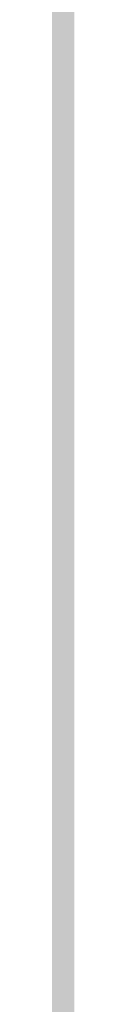
# Model space of a CAD drawing. Units: inches. Extents: x 2083 to 3317, y 1141 to 2115.
# Tile 191 of 256: x 3126.9559 to 3126.9582, y 1263.3548 to 1263.6134. Entities that reach past the tile are written whole.
import ezdxf

# ---------------------------------------------------------------- set-up
doc = ezdxf.new("R2010")
doc.units = ezdxf.units.IN
doc.layers.add('A-ANNO-DIMS', color=2, linetype='Continuous', lineweight=18)
doc.layers.add('A-WALL-PATT', color=251, linetype='Continuous', lineweight=13, true_color=0x636466)
doc.styles.get("Standard").update_dxf_attribs({"font": 'arial.ttf'})
doc.dimstyles.new('ISO-25', dxfattribs={"dimtxt": 12, "dimasz": 12, "dimexe": 1.25, "dimexo": 0.625, "dimtad": 1, "dimlunit": 3, "dimtxsty": 'Standard', "dimcen": 2.5, "dimadec": 0, "dimazin": 0, "dimtfac": 1, "dimtmove": 0, "dimatfit": 3, "dimfxl": 1, "dimarcsym": 0})

# ---------------------------------------------------------------- blocks, each defined once
blk = doc.blocks.new('*D26')
at = {"layer": 'A-ANNO-DIMS', "color": 0, "lineweight": -2, "transparency": 16777216}
for p, q in [((3088.98584, 1274.91509), (3088.98584, 1270.95196)), ((3111.24004, 1274.91509), (3111.24004, 1270.95196)), ((3076.98584, 1272.20196), (2840.26245, 1272.20196)), ((3111.24004, 1272.20196), (3088.98584, 1272.20196)), ((3123.24004, 1272.20196), (3135.24004, 1272.20196))]:
    blk.add_line(p, q, dxfattribs=at)
at = {"layer": 'A-ANNO-DIMS', "color": 0, "transparency": 16777216}
for points in [[(3076.98584, 1274.20196), (3076.98584, 1270.20196), (3088.98584, 1272.20196)], [(3123.24004, 1274.20196), (3123.24004, 1270.20196), (3111.24004, 1272.20196)]]:
    blk.add_solid(points, dxfattribs=at)
at = {"layer": 'Defpoints', "color": 0, "transparency": 16777216}
for p in [(3088.98584, 1275.54009), (3111.24004, 1275.54009), (3088.98584, 1272.20196)]:
    blk.add_point(p, dxfattribs=at)
at = {"layer": 'A-ANNO-DIMS', "color": 0, "transparency": 16777216, "insert": (2952.62415, 1279.0316), "char_height": 12, "attachment_point": 5}
blk.add_mtext('NIGHTSTAND 1\'-10 1/2" TYP.', dxfattribs=at)
blk = doc.blocks.new('*D27')
at = {"layer": 'A-ANNO-DIMS', "color": 0, "lineweight": -2, "transparency": 16777216}
for p, q in [((3114.57817, 1309.79428), (3114.57817, 1321.79428)), ((3111.86504, 1297.79428), (3115.82817, 1297.79428)), ((3114.57817, 1297.79428), (3114.57817, 1275.54009)), ((3111.86504, 1275.54009), (3115.82817, 1275.54009)), ((3114.57817, 1263.54009), (3114.57817, 1140.98859))]:
    blk.add_line(p, q, dxfattribs=at)
at = {"layer": 'A-ANNO-DIMS', "color": 0, "transparency": 16777216}
for points in [[(3112.57817, 1309.79428), (3116.57817, 1309.79428), (3114.57817, 1297.79428)], [(3112.57817, 1263.54009), (3116.57817, 1263.54009), (3114.57817, 1275.54009)]]:
    blk.add_solid(points, dxfattribs=at)
at = {"layer": 'Defpoints', "color": 0, "transparency": 16777216}
for p in [(3111.24004, 1297.79428), (3111.24004, 1275.54009), (3114.57817, 1275.54009)]:
    blk.add_point(p, dxfattribs=at)
at = {"layer": 'A-ANNO-DIMS', "color": 0, "transparency": 16777216, "insert": (3107.74853, 1196.26434), "char_height": 12, "attachment_point": 5, "rotation": 90}
blk.add_mtext('1\'-10 1/2" TYP.', dxfattribs=at)

msp = doc.modelspace()

# ---------------------------------------------------------------- hatches: boundary and pattern name
at = {"layer": 'A-WALL-PATT'}
h = msp.add_hatch(color=256, dxfattribs=at)
h.dxf.hatch_style = 1
h.paths.add_polyline_path([(3126.95978, 2020.76136), (2748.95978, 2020.76136), (2604.95978, 2020.76136), (2226.95978, 2020.76136), (2226.95978, 1702.76136), (2466.95978, 1702.76136), (2466.95978, 1582.76136), (2418.95978, 1582.76136), (2418.95978, 1477.76136), (2226.95978, 1477.76136), (2226.95978, 1263.26136), (2544.95978, 1263.26136), (2544.95978, 1411.76136), (2604.95978, 1411.76136), (2685.95978, 1411.76136), (2685.95978, 1420.76136), (2604.95978, 1420.76136), (2604.95978, 1573.76136), (2604.95978, 1702.76136), (2604.95978, 2011.76136), (2748.95978, 2011.76136), (2748.95978, 1702.76136), (2862.95978, 1702.76136), (2862.95978, 1621.76136), (2871.95978, 1621.76136), (2871.95978, 1702.76136), (2883.95978, 1702.76136), (2883.95978, 1706.93946, -0.026459), (2883.95978, 1711.76136), (2757.95978, 1711.76136), (2757.95978, 1807.76136), (2787.95978, 1807.76136), (2787.95978, 1812.26136), (2757.95978, 1812.26136), (2757.95978, 2011.76136), (2877.95978, 2011.76136), (2877.95978, 1812.26136), (2847.95978, 1812.26136), (2847.95978, 1807.76136), (2889.83574, 1807.76136), (2889.83574, 1812.26136), (2882.45978, 1812.26136), (2882.45978, 2011.76136), (3117.95978, 2011.76136), (3117.95978, 1812.26136), (2937.83574, 1812.26136), (2937.83574, 1807.76136), (2995.70978, 1807.76136), (2995.70978, 1796.11767), (3000.20978, 1796.11767), (3000.20978, 1807.76136), (3117.95978, 1807.76136), (3117.95978, 1711.76136), (3000.20978, 1711.76136), (3000.20978, 1760.11767), (2998.5727, 1760.11767, -0.020711), (2995.70978, 1760.11767), (2995.70978, 1711.76136), (2931.95978, 1711.76136), (2931.95978, 1702.76136), (3126.95978, 1702.76136)])
h.paths.add_polyline_path([(2471.45978, 2011.76136), (2471.45978, 1810.01136), (2462.71694, 1810.01136), (2462.71694, 1805.51136), (2505.95978, 1805.51136), (2505.95978, 1810.01136), (2475.95978, 1810.01136), (2475.95978, 2011.76136), (2595.95978, 2011.76136), (2595.95978, 1810.01136), (2565.95978, 1810.01136), (2565.95978, 1805.51136), (2595.95978, 1805.51136), (2595.95978, 1711.76136), (2235.95978, 1711.76136), (2235.95978, 1805.51136), (2353.70978, 1805.51136), (2353.70978, 1796.05416), (2358.20978, 1796.05416), (2358.20978, 1805.51136), (2414.71694, 1805.51136), (2414.71694, 1810.01136), (2235.95978, 1810.01136), (2235.95978, 2011.76136)], flags=16)
h.paths.add_polyline_path([(2270.20473, 1994.61001), (2270.20473, 1970.61001), (2246.20473, 1970.61001), (2246.20473, 1994.61001)], flags=0)
edge = h.paths.add_edge_path(flags=0)
edge.add_ellipse((2332.02739, 1899.79818), major_axis=(-3.04299, 3.04299), ratio=0.1682525, start_angle=-161.33217, end_angle=-156.30711, ccw=False)
edge.add_ellipse((2333.08204, 1898.74353), major_axis=(-1.05465, 1.05465), ratio=0.4535321, start_angle=-123.37102, end_angle=-94.15911)
edge = h.paths.add_edge_path(flags=0)
edge.add_ellipse((2332.02739, 1968.87629), major_axis=(3.04299, 3.04299), ratio=0.1682525, start_angle=18.66783, end_angle=23.69289)
edge.add_spline(control_points=[(2332.9256, 1970.6911), (2332.22677, 1970.3361), (2330.89371, 1969.65891), (2328.41308, 1970.93214), (2327.20393, 1967.74871), (2324.7096, 1969.95559), (2322.53282, 1967.01235), (2320.01285, 1971.29581), (2317.68031, 1968.15784), (2316.04053, 1967.10205), (2315.4269, 1966.8096)], knot_values=[0, 0, 0, 0, 2.267059, 4.324559, 6.685584, 8.878641, 11.121502, 14.300359, 17.755284, 19.732645, 19.732645, 19.732645, 19.732645], degree=3, periodic=0)
edge.add_ellipse((2332.02739, 1968.87629), major_axis=(3.04299, 3.04299), ratio=0.1682525, start_angle=18.66783, end_angle=23.69289, ccw=False)
edge.add_ellipse((2333.08204, 1969.93094), major_axis=(1.05465, 1.05465), ratio=0.4535321, start_angle=56.62898, end_angle=85.84089, ccw=False)
edge = h.paths.add_edge_path(flags=0)
edge.add_spline(control_points=[(2296.42829, 1967.98791), (2293.6278, 1965.33631), (2287.70362, 1959.72709), (2299.74386, 1949.9957), (2294.53259, 1935.66853), (2290.57323, 1920.60351), (2293.39412, 1909.97369), (2296.18541, 1904.96654)], knot_values=[0.099185, 0.099185, 0.099185, 0.099185, 0.345301, 0.619822, 0.982653, 1.386093, 1.810555, 1.810555, 1.810555, 1.810555], degree=3, periodic=0)
edge.add_spline(control_points=[(2296.18541, 1904.96654), (2297.38358, 1902.6193), (2298.00097, 1901.94931), (2298.55297, 1901.46815)], knot_values=[0.006246, 0.006246, 0.006246, 0.006246, 0.055476, 0.055476, 0.055476, 0.055476], degree=3, periodic=0)
edge.add_spline(control_points=[(2298.55297, 1901.46815), (2297.25861, 1900.92322), (2295.22529, 1900.23213), (2293.06023, 1900.61421), (2292.10142, 1900.78841), (2292.08958, 1900.79057)], knot_values=[0.312835, 0.312835, 0.312835, 0.312835, 0.40178, 0.474987, 0.475903, 0.475903, 0.475903, 0.475903], degree=3, periodic=0)
edge.add_arc((2292.79365, 1904.66411), 3.93701, 215.4209, 259.69818, ccw=False)
edge.add_spline(control_points=[(2289.58531, 1902.3823), (2289.47665, 1902.53509), (2289.36848, 1902.68804), (2289.26086, 1902.84117)], knot_values=[0.102872, 0.102872, 0.102872, 0.102872, 0.116896, 0.116896, 0.116896, 0.116896], degree=3, periodic=0)
edge.add_spline(control_points=[(2289.26086, 1902.84117), (2288.6866, 1902.55019), (2287.64005, 1902.0199), (2285.88134, 1901.87395), (2283.85297, 1901.50435), (2281.71999, 1899.71054), (2278.46699, 1899.49294), (2276.15714, 1901.8832), (2272.25895, 1899.80407), (2267.77761, 1901.84318), (2262.24388, 1900.18403), (2257.41493, 1901.78206), (2254.31837, 1900.72612), (2253.17828, 1900.33734)], knot_values=[0, 0, 0, 0, 1.907977, 3.477176, 5.261074, 7.972851, 11.680248, 13.717921, 16.939592, 22.789562, 27.502503, 33.595215, 37.145618, 37.145618, 37.145618, 37.145618], degree=3, periodic=0)
edge.add_line((2253.17828, 1900.33734), (2250.24424, 1902.84117))
edge.add_line((2250.24424, 1902.84117), (2250.24424, 1965.8333))
edge.add_line((2250.24424, 1965.8333), (2253.17828, 1968.33712))
edge.add_spline(control_points=[(2253.17828, 1968.33712), (2254.31837, 1967.94835), (2257.41493, 1966.89241), (2262.24388, 1968.49043), (2267.77761, 1966.83128), (2271.52673, 1968.53722), (2273.87591, 1967.82829), (2274.2067, 1967.72764)], knot_values=[0, 0, 0, 0, 0.09018, 0.244935, 0.364644, 0.513233, 0.537855, 0.537855, 0.537855, 0.537855], degree=3, periodic=0)
edge.add_arc((2274.35289, 1963.79335), 3.93701, 72.05113, 92.12795, ccw=False)
edge.add_arc((2281.29693, 1985.23), 18.5963, 252.051134, 288.565722)
edge.add_arc((2292.31672, 1956.02888), 12.64608, 71.026788, 113.778218, ccw=False)
edge = h.paths.add_edge_path(flags=0)
edge.add_spline(control_points=[(2274.89941, 1951.85619), (2275.06616, 1951.61659), (2275.23269, 1951.37659), (2275.39799, 1951.13585)], knot_values=[1.409916, 1.409916, 1.409916, 1.409916, 1.43159, 1.43159, 1.43159, 1.43159], degree=3, periodic=0)
edge.add_spline(control_points=[(2275.39799, 1951.13585), (2275.79211, 1950.56189), (2276.17923, 1949.98377), (2276.54555, 1949.3971)], knot_values=[1.358238, 1.358238, 1.358238, 1.358238, 1.409916, 1.409916, 1.409916, 1.409916], degree=3, periodic=0)
edge.add_line((2276.54555, 1949.3971), (2277.43729, 1947.86218))
edge.add_spline(control_points=[(2277.43729, 1947.86218), (2276.30383, 1945.67311), (2274.6397, 1942.42688), (2274.63161, 1938.0939), (2272.79912, 1930.85155), (2274.35643, 1943.89705), (2275.94768, 1947.92336), (2276.54555, 1949.3971)], knot_values=[0.005632, 0.005632, 0.005632, 0.005632, 0.186014, 0.266002, 0.357087, 0.59639, 0.739732, 0.739732, 0.739732, 0.739732], degree=3, periodic=0)
edge.add_spline(control_points=[(2276.54555, 1949.3971), (2276.17923, 1949.98377), (2275.79211, 1950.56189), (2275.39799, 1951.13585)], knot_values=[1.358238, 1.358238, 1.358238, 1.358238, 1.409916, 1.409916, 1.409916, 1.409916], degree=3, periodic=0)
edge.add_spline(control_points=[(2275.39799, 1951.13585), (2274.9425, 1950.08045), (2274.20776, 1948.02527), (2273.9346, 1944.85148), (2272.46853, 1937.62749), (2273.46622, 1945.69647), (2274.70062, 1951.05947), (2274.89941, 1951.85619)], knot_values=[0.104364, 0.104364, 0.104364, 0.104364, 0.189636, 0.269624, 0.36071, 0.600013, 0.644622, 0.644622, 0.644622, 0.644622], degree=3, periodic=0)
h.paths.add_polyline_path([(2269.16751, 1963.12757, -0.357527), (2268.17063, 1960.97637, -0.092561), (2268.17063, 1939.43632, -0.357527), (2269.16751, 1937.28512, -0.357527), (2267.01631, 1938.282, -0.164785), (2254.68558, 1938.282, -0.357527), (2252.53438, 1937.28512, -0.357527), (2253.53126, 1939.43632, -0.092561), (2253.53126, 1960.97637, -0.357527), (2252.53438, 1963.12757, -0.357527), (2254.68558, 1962.13069, -0.164785), (2267.01631, 1962.13069, -0.357527)], flags=0)
h.paths.add_polyline_path([(2248.87407, 1967.8018), (2248.87407, 1957.02771), (2249.45778, 1957.02771), (2249.45778, 1911.64676), (2248.87407, 1911.64676), (2248.87407, 1900.87267), (2246.51186, 1900.87267, 0.197327), (2244.14966, 1902.45687), (2244.14966, 1966.21759, 0.197327), (2246.51186, 1967.8018)], flags=0)
h.paths.add_polyline_path([(2269.16751, 1931.38934, -0.357527), (2268.17063, 1929.23814, -0.092561), (2268.17063, 1907.6981, -0.357527), (2269.16751, 1905.54689, -0.357527), (2267.01631, 1906.54377, -0.164785), (2254.68558, 1906.54377, -0.357527), (2252.53438, 1905.54689, -0.357527), (2253.53126, 1907.6981, -0.092561), (2253.53126, 1929.23814, -0.357527), (2252.53438, 1931.38934, -0.357527), (2254.68558, 1930.39246, -0.164785), (2267.01631, 1930.39246, -0.357527)], flags=0)
edge = h.paths.add_edge_path(flags=0)
edge.add_spline(control_points=[(2276.19686, 1906.7237), (2276.16814, 1909.02893), (2276.11405, 1913.37185), (2270.59842, 1924.92498), (2273.90517, 1919.01278), (2275.92171, 1916.26206), (2275.47457, 1912.40215), (2277.25787, 1910.38062), (2276.69604, 1908.22504), (2276.64622, 1906.81302), (2276.61782, 1906.00841)], knot_values=[0, 0, 0, 0, 8.61026, 16.221274, 18.843057, 23.804898, 27.440828, 29.356102, 31.203478, 33.650687, 33.650687, 33.650687, 33.650687], degree=3, periodic=0)
edge.add_spline(control_points=[(2276.61782, 1906.00841), (2276.62331, 1905.62414), (2276.49774, 1904.62866), (2275.44178, 1903.85473), (2274.93731, 1903.08045), (2274.85908, 1902.84117)], knot_values=[0.156488, 0.156488, 0.156488, 0.156488, 0.184398, 0.231376, 0.250598, 0.250598, 0.250598, 0.250598], degree=3, periodic=0)
edge.add_line((2274.85908, 1902.84117), (2276.50598, 1902.84117))
edge.add_spline(control_points=[(2276.50598, 1902.84117), (2276.78831, 1903.08494), (2277.66507, 1904.1252), (2278.24954, 1904.34074), (2277.65387, 1908.52739), (2278.15567, 1906.22781), (2278.10046, 1905.28595), (2278.84667, 1904.06901), (2277.85679, 1903.41495), (2277.87419, 1902.99105), (2277.90356, 1902.84117)], knot_values=[0.059574, 0.059574, 0.059574, 0.059574, 0.080753, 0.103741, 0.16972, 0.176036, 0.207137, 0.240474, 0.262341, 0.27366, 0.27366, 0.27366, 0.27366], degree=3, periodic=0)
edge.add_line((2277.90356, 1902.84117), (2280.02983, 1902.84117))
edge.add_spline(control_points=[(2280.02983, 1902.84117), (2279.88822, 1903.0884), (2279.49926, 1903.98155), (2280.15228, 1905.93935), (2278.10362, 1909.65776), (2279.76239, 1907.18529), (2280.3279, 1904.87486), (2280.48511, 1903.48959), (2281.46327, 1903.24943), (2281.75834, 1902.9365), (2281.83404, 1902.84117)], knot_values=[0.013856, 0.013856, 0.013856, 0.013856, 0.034874, 0.088867, 0.107879, 0.126738, 0.158714, 0.193757, 0.217487, 0.226722, 0.226722, 0.226722, 0.226722], degree=3, periodic=0)
edge.add_spline(control_points=[(2281.83404, 1902.84117), (2281.78753, 1902.8267), (2281.64702, 1902.78299), (2281.39553, 1902.85949), (2281.08808, 1902.98524), (2280.72068, 1903.0609), (2280.33345, 1903.02573), (2280.12477, 1902.89888), (2280.02983, 1902.84117)], knot_values=[0, 0, 0, 0, 0.14413, 0.435517, 0.749276, 1.153046, 1.548371, 1.878348, 1.878348, 1.878348, 1.878348], degree=3, periodic=0)
edge.add_line((2280.02983, 1902.84117), (2277.90356, 1902.84117))
edge.add_spline(control_points=[(2277.90356, 1902.84117), (2277.89286, 1902.79586), (2277.8654, 1902.67964), (2277.60748, 1902.68748), (2277.27405, 1902.8007), (2276.83792, 1902.61977), (2276.58381, 1902.78926), (2276.50598, 1902.84117)], knot_values=[0, 0, 0, 0, 0.127189, 0.326199, 0.628009, 1.24357, 1.515331, 1.515331, 1.515331, 1.515331], degree=3, periodic=0)
edge.add_line((2276.50598, 1902.84117), (2274.85908, 1902.84117))
edge.add_spline(control_points=[(2274.85908, 1902.84117), (2274.81444, 1902.89859), (2274.72513, 1903.01345), (2274.49348, 1903.11897), (2274.24429, 1902.96054), (2273.93712, 1903.18494), (2273.61404, 1902.98314), (2273.40832, 1902.88304), (2273.32225, 1902.84117)], knot_values=[0, 0, 0, 0, 0.21843, 0.436957, 0.687977, 0.990379, 1.398396, 1.69185, 1.69185, 1.69185, 1.69185], degree=3, periodic=0)
edge.add_spline(control_points=[(2273.32225, 1902.84117), (2273.61674, 1903.44569), (2274.274, 1904.53825), (2276.02724, 1904.5737), (2276.20696, 1906.58364), (2276.19686, 1906.7237)], knot_values=[0.012227, 0.012227, 0.012227, 0.012227, 0.059472, 0.106218, 0.134458, 0.134458, 0.134458, 0.134458], degree=3, periodic=0)
h.paths.add_polyline_path([(2270.77605, 1897.78983), (2270.77605, 1873.78983), (2246.77605, 1873.78983), (2246.77605, 1897.78983)], flags=0)
h.paths.add_polyline_path([(2353.70978, 1760.00506), (2353.70978, 1760.05416), (2358.20978, 1760.05416, -0.033729)], flags=0)
h.paths.add_polyline_path([(2321.81912, 1737.52919), (2341.99533, 1737.52919, -0.414214), (2343.20327, 1736.32124), (2343.20327, 1721.0206, -0.414214), (2341.99533, 1719.81265), (2321.81912, 1719.81265, -0.414214), (2320.61117, 1721.0206), (2320.61117, 1736.32124, -0.414214)], flags=0)
h.paths.add_polyline_path([(2324.23501, 1736.32124), (2339.57944, 1736.32124, -0.414214), (2341.99533, 1733.90535), (2341.99533, 1725.44973, -0.414214), (2339.57944, 1723.03384), (2333.68059, 1723.03384), (2333.84532, 1722.04547, -0.870646), (2335.4254, 1721.82589, -0.767327), (2333.92269, 1721.42324), (2331.29102, 1721.42324, -0.767327), (2329.78832, 1721.82589, -0.870646), (2331.3684, 1722.04547), (2331.53313, 1723.03384), (2324.23501, 1723.03384, -0.414214), (2321.81912, 1725.44973), (2321.81912, 1733.90535, -0.414214)], flags=0)
h.paths.add_polyline_path([(2570.48379, 1928.61544), (2589.68379, 1928.61544), (2590.16883, 1928.61544), (2590.16883, 1904.9934), (2570.48379, 1904.9934)], flags=0)
h.paths.add_polyline_path([(2574.44732, 1927.26382, -1), (2572.82884, 1927.26382, -1)], flags=0)
h.paths.add_polyline_path([(2573.08987, 1926.94088), (2573.92503, 1927.77604), (2574.14774, 1927.55333), (2573.31258, 1926.71817)], flags=0)
h.paths.add_polyline_path([(2578.77906, 1919.72962, -1), (2571.59166, 1919.72962, -1)], flags=0)
h.paths.add_polyline_path([(2578.38536, 1919.72962, -1), (2571.98536, 1919.72962, -1)], flags=0)
h.paths.add_polyline_path([(2331.59576, 1729.47622, -1), (2333.61795, 1729.47622, -1)], flags=0)
h.paths.add_polyline_path([(2578.03423, 1927.26382, -1), (2576.41574, 1927.26382, -1)], flags=0)
h.paths.add_polyline_path([(2576.68885, 1927.53109), (2576.91156, 1927.7538), (2577.74673, 1926.91863), (2577.52402, 1926.69592)], flags=0)
h.paths.add_polyline_path([(2578.13906, 1909.85954, -1), (2572.23166, 1909.85954, -1)], flags=0)
h.paths.add_polyline_path([(2577.74536, 1909.85954, -1), (2572.62536, 1909.85954, -1)], flags=0)
h.paths.add_polyline_path([(2583.79772, 1927.26382, -1), (2582.17923, 1927.26382, -1)], flags=0)
h.paths.add_polyline_path([(2582.71865, 1927.7538), (2583.55381, 1926.91863), (2583.3311, 1926.69592), (2582.49594, 1927.53109)], flags=0)
h.paths.add_polyline_path([(2582.49594, 1927.53109), (2582.71865, 1927.7538), (2583.55381, 1926.91863), (2583.3311, 1926.69592)], flags=0)
h.paths.add_polyline_path([(2587.73906, 1920.52962, -1), (2581.83166, 1920.52962, -1)], flags=0)
h.paths.add_polyline_path([(2587.34536, 1920.52962, -1), (2582.22536, 1920.52962, -1)], flags=0)
h.paths.add_polyline_path([(2587.38462, 1927.26382, -1), (2585.76613, 1927.26382, -1)], flags=0)
h.paths.add_polyline_path([(2586.08199, 1926.98025), (2586.91716, 1927.81541), (2587.13987, 1927.5927), (2586.3047, 1926.75754)], flags=0)
h.paths.add_polyline_path([(2588.37906, 1910.65954, -1), (2581.19166, 1910.65954, -1)], flags=0)
h.paths.add_polyline_path([(2587.98536, 1910.65954, -1), (2581.58536, 1910.65954, -1)], flags=0)
h.paths.add_polyline_path([(2417.16773, 1729.4779), (2437.34394, 1729.4779, -0.414214), (2438.55188, 1728.26995), (2438.55188, 1712.96931, -0.414214), (2437.34394, 1711.76136), (2417.16773, 1711.76136, -0.414214), (2415.95978, 1712.96931), (2415.95978, 1728.26995, -0.414214)], flags=0)
h.paths.add_polyline_path([(2419.58362, 1728.26995), (2434.92805, 1728.26995, -0.414214), (2437.34394, 1725.85406), (2437.34394, 1717.39844, -0.414214), (2434.92805, 1714.98255), (2429.0292, 1714.98255), (2429.19393, 1713.99418, -0.870646), (2430.77401, 1713.7746, -0.767327), (2429.2713, 1713.37195), (2426.63963, 1713.37195, -0.767327), (2425.13693, 1713.7746, -0.870646), (2426.71701, 1713.99418), (2426.88174, 1714.98255), (2419.58362, 1714.98255, -0.414214), (2417.16773, 1717.39844), (2417.16773, 1725.85406, -0.414214)], flags=0)
h.paths.add_polyline_path([(2419.58362, 1728.26995), (2434.92805, 1728.26995, -0.414214), (2437.34394, 1725.85406), (2437.34394, 1717.39844, -0.414214), (2434.92805, 1714.98255), (2429.0292, 1714.98255), (2428.35812, 1719.00903), (2427.55282, 1719.00903), (2426.88174, 1714.98255), (2419.58362, 1714.98255, -0.414214), (2417.16773, 1717.39844), (2417.16773, 1725.85406, -0.414214)], flags=0)
h.paths.add_polyline_path([(2426.94437, 1721.42492, -1), (2428.96656, 1721.42492, -1)], flags=0)
h.paths.add_polyline_path([(2475.95978, 1702.76136), (2595.95978, 1702.76136), (2595.95978, 1582.76136), (2475.95978, 1582.76136)], flags=16)
h.paths.add_polyline_path([(2427.95978, 1573.76136), (2595.95978, 1573.76136), (2595.95978, 1468.76136), (2595.95978, 1420.76136), (2384.45978, 1420.76136), (2384.45978, 1468.76136), (2427.95978, 1468.76136)], flags=16)
h.paths.add_polyline_path([(2379.95978, 1468.76136), (2379.95978, 1420.76136), (2235.95978, 1420.76136), (2235.95978, 1468.76136)], flags=16)
h.paths.add_polyline_path([(2317.816, 1466.69577), (2337.9922, 1466.69577, -0.414214), (2339.20015, 1465.48782), (2339.20015, 1450.18718, -0.414214), (2337.9922, 1448.97923), (2317.816, 1448.97923, -0.414214), (2316.60805, 1450.18718), (2316.60805, 1465.48782, -0.414214)], flags=0)
h.paths.add_polyline_path([(2320.23189, 1465.48782), (2335.57631, 1465.48782, -0.414214), (2337.9922, 1463.07193), (2337.9922, 1454.61631, -0.414214), (2335.57631, 1452.20042), (2329.67747, 1452.20042), (2329.84219, 1451.21205, -0.870646), (2331.42228, 1450.99247, -0.767327), (2329.91957, 1450.58983), (2327.2879, 1450.58983, -0.767327), (2325.7852, 1450.99247, -0.870646), (2327.36528, 1451.21205), (2327.53001, 1452.20042), (2320.23189, 1452.20042, -0.414214), (2317.816, 1454.61631), (2317.816, 1463.07193, -0.414214)], flags=0)
h.paths.add_polyline_path([(2320.23189, 1465.48782), (2335.57631, 1465.48782, -0.414214), (2337.9922, 1463.07193), (2337.9922, 1454.61631, -0.414214), (2335.57631, 1452.20042), (2329.67747, 1452.20042), (2329.00638, 1456.22691), (2328.20109, 1456.22691), (2327.53001, 1452.20042), (2320.23189, 1452.20042, -0.414214), (2317.816, 1454.61631), (2317.816, 1463.07193, -0.414214)], flags=0)
h.paths.add_polyline_path([(2327.59264, 1458.6428, -1), (2329.61483, 1458.6428, -1)], flags=0)
h.paths.add_polyline_path([(2244.41174, 1433.34045), (2241.92094, 1433.34045, -0.414214), (2240.01786, 1435.24354), (2240.01786, 1440.95281, -0.414211), (2241.92093, 1442.8559), (2244.41174, 1442.8559, -1.976472)], flags=0)
h.paths.add_polyline_path([(2245.35689, 1434.39754, -0.414214), (2245.35689, 1441.79881, -2.144098)], flags=0)
h.paths.add_polyline_path([(2535.95978, 1416.26136), (2535.95978, 1272.26136), (2235.95978, 1272.26136), (2235.95978, 1416.26136)], flags=16)
h.paths.add_polyline_path([(2260.11956, 1384.29284), (2260.11956, 1362.03865), (2237.86537, 1362.03865), (2237.86537, 1384.29284)], flags=0)
edge = h.paths.add_edge_path(flags=0)
edge.add_line((2318.25185, 1362.0933), (2318.1458, 1362.00097))
edge.add_ellipse((2317.44512, 1360.43104), major_axis=(2.82164, 2.82164), ratio=0.1682525, start_angle=18.66783, end_angle=20.94813, ccw=False)
edge.add_ellipse((2318.42305, 1361.40897), major_axis=(0.97793, 0.97793), ratio=0.4535321, start_angle=56.62898, end_angle=70.2262, ccw=False)
edge = h.paths.add_edge_path(flags=0)
edge.add_line((2319.10737, 1295.57108), (2319.01504, 1295.67713))
edge.add_ellipse((2317.44512, 1296.37781), major_axis=(-2.82164, 2.82164), ratio=0.1682525, start_angle=-161.33217, end_angle=-159.05187, ccw=False)
edge.add_ellipse((2318.42305, 1295.39988), major_axis=(-0.97793, 0.97793), ratio=0.4535321, start_angle=-123.37102, end_angle=-109.7738)
edge = h.paths.add_edge_path(flags=0)
edge.add_spline(control_points=[(2284.21035, 1301.17022), (2284.58069, 1300.44472), (2284.89119, 1299.89202), (2285.15955, 1299.46102)], knot_values=[0.039066, 0.039066, 0.039066, 0.039066, 0.055476, 0.055476, 0.055476, 0.055476], degree=3, periodic=0)
edge.add_line((2285.15955, 1299.46102), (2284.21035, 1301.17022))
edge = h.paths.add_edge_path(flags=0)
edge.add_line((2280.41246, 1297.29801), (2283.36999, 1297.03612))
edge.add_line((2283.36999, 1297.03612), (2286.40569, 1297.92631))
edge.add_spline(control_points=[(2286.40569, 1297.92631), (2285.30549, 1297.46312), (2284.34478, 1297.12915), (2283.36999, 1297.03612)], knot_values=[0.394369, 0.394369, 0.394369, 0.394369, 0.475903, 0.475903, 0.475903, 0.475903], degree=3, periodic=0)
edge.add_spline(control_points=[(2283.36999, 1297.03612), (2283.28139, 1297.02767), (2282.31629, 1296.95734), (2281.3125, 1297.13448), (2280.42344, 1297.29602), (2280.41246, 1297.29801)], knot_values=[0.312835, 0.312835, 0.312835, 0.312835, 0.320246, 0.393453, 0.394369, 0.394369, 0.394369, 0.394369], degree=3, periodic=0)
edge = h.paths.add_edge_path(flags=0)
edge.add_line((2284.43556, 1359.60729), (2280.44629, 1355.32805))
edge.add_line((2280.44629, 1355.32805), (2279.57999, 1351.01775))
edge.add_line((2279.57999, 1351.01775), (2282.41297, 1346.58043))
edge.add_spline(control_points=[(2282.41297, 1346.58043), (2283.15333, 1345.58924), (2284.2529, 1344.0289), (2284.80104, 1342.38717), (2284.93516, 1341.80554)], knot_values=[1.240098, 1.240098, 1.240098, 1.240098, 1.332892, 1.382712, 1.382712, 1.382712, 1.382712], degree=3, periodic=0)
edge.add_spline(control_points=[(2284.93516, 1341.80554), (2285.31911, 1340.1406), (2285.23303, 1338.4092), (2284.90994, 1336.65412)], knot_values=[1.097484, 1.097484, 1.097484, 1.097484, 1.240098, 1.240098, 1.240098, 1.240098], degree=3, periodic=0)
edge.add_spline(control_points=[(2284.90994, 1336.65412), (2284.58685, 1334.89904), (2284.02675, 1333.12027), (2283.46264, 1331.36058)], knot_values=[0.95487, 0.95487, 0.95487, 0.95487, 1.097484, 1.097484, 1.097484, 1.097484], degree=3, periodic=0)
edge.add_line((2283.46264, 1331.36058), (2281.89038, 1326.15336))
edge.add_line((2281.89038, 1326.15336), (2280.75626, 1321.05609))
edge.add_line((2280.75626, 1321.05609), (2280.2992, 1316.00198))
edge.add_line((2280.2992, 1316.00198), (2280.71593, 1310.95007))
edge.add_line((2280.71593, 1310.95007), (2282.02809, 1305.97214))
edge.add_line((2282.02809, 1305.97214), (2284.21035, 1301.17022))
edge.add_spline(control_points=[(2284.21035, 1301.17022), (2283.34073, 1302.73019), (2282.6119, 1304.33649), (2282.02809, 1305.97214)], knot_values=[0.099185, 0.099185, 0.099185, 0.099185, 0.241799, 0.241799, 0.241799, 0.241799], degree=3, periodic=0)
edge.add_spline(control_points=[(2282.02809, 1305.97214), (2281.44428, 1307.60778), (2281.00549, 1309.27276), (2280.71593, 1310.95007)], knot_values=[0.241799, 0.241799, 0.241799, 0.241799, 0.384413, 0.384413, 0.384413, 0.384413], degree=3, periodic=0)
edge.add_spline(control_points=[(2280.71593, 1310.95007), (2280.43324, 1312.58761), (2280.28939, 1314.27696), (2280.29889, 1315.96203), (2280.2992, 1316.00198)], knot_values=[0.384413, 0.384413, 0.384413, 0.384413, 0.523647, 0.527028, 0.527028, 0.527028, 0.527028], degree=3, periodic=0)
edge.add_spline(control_points=[(2280.2992, 1316.00198), (2280.31233, 1317.68696), (2280.47787, 1319.36793), (2280.75626, 1321.05609)], knot_values=[0.527028, 0.527028, 0.527028, 0.527028, 0.669642, 0.669642, 0.669642, 0.669642], degree=3, periodic=0)
edge.add_spline(control_points=[(2280.75626, 1321.05609), (2281.03465, 1322.74425), (2281.42588, 1324.43961), (2281.89038, 1326.15336)], knot_values=[0.669642, 0.669642, 0.669642, 0.669642, 0.812256, 0.812256, 0.812256, 0.812256], degree=3, periodic=0)
edge.add_spline(control_points=[(2281.89038, 1326.15336), (2282.26438, 1327.53325), (2282.78787, 1329.26181), (2283.35275, 1331.01778), (2283.46264, 1331.36058)], knot_values=[0.812256, 0.812256, 0.812256, 0.812256, 0.927087, 0.95487, 0.95487, 0.95487, 0.95487], degree=3, periodic=0)
edge.add_line((2283.46264, 1331.36058), (2284.90994, 1336.65412))
edge.add_line((2284.90994, 1336.65412), (2284.93516, 1341.80554))
edge.add_line((2284.93516, 1341.80554), (2282.41297, 1346.58043))
edge.add_spline(control_points=[(2282.41297, 1346.58043), (2281.27513, 1348.10379), (2280.07845, 1349.57032), (2279.57999, 1351.01775)], knot_values=[1.382712, 1.382712, 1.382712, 1.382712, 1.525326, 1.525326, 1.525326, 1.525326], degree=3, periodic=0)
edge.add_spline(control_points=[(2279.57999, 1351.01775), (2279.44328, 1351.41472), (2279.13631, 1352.85692), (2279.73519, 1354.29039), (2280.44629, 1355.32805)], knot_values=[1.525326, 1.525326, 1.525326, 1.525326, 1.564439, 1.667941, 1.667941, 1.667941, 1.667941], degree=3, periodic=0)
edge.add_spline(control_points=[(2280.44629, 1355.32805), (2281.42611, 1356.75784), (2282.93084, 1358.18256), (2284.43556, 1359.60729)], knot_values=[1.667941, 1.667941, 1.667941, 1.667941, 1.810555, 1.810555, 1.810555, 1.810555], degree=3, periodic=0)
edge.add_arc((2280.62307, 1348.51818), 11.72618, 71.026788, 113.778218)
edge.add_arc((2270.40489, 1375.59516), 17.24357, 252.051134, 288.565722, ccw=False)
edge.add_arc((2263.96597, 1355.71785), 3.65062, 72.05113, 92.12795)
edge.add_arc((2263.96597, 1355.71785), 3.65062, 92.12795, 177.98513)
edge.add_spline(control_points=[(2260.3176, 1355.8462), (2260.26042, 1354.22067), (2260.55128, 1350.18655), (2262.99934, 1346.76625), (2264.47274, 1344.64902)], knot_values=[1.43159, 1.43159, 1.43159, 1.43159, 1.564144, 1.770695, 1.770695, 1.770695, 1.770695], degree=3, periodic=0)
edge.add_line((2264.47274, 1344.64902), (2264.93559, 1343.98253))
edge.add_spline(control_points=[(2263.80104, 1340.24811), (2263.84324, 1340.51409), (2264.06724, 1341.75647), (2264.51269, 1343.00245), (2264.93505, 1343.98108)], knot_values=[0.53657, 0.53657, 0.53657, 0.53657, 0.559349, 0.644622, 0.644622, 0.644622, 0.644622], degree=3, periodic=0)
edge.add_spline(control_points=[(2264.93505, 1343.98108), (2265.11777, 1343.71497), (2265.29888, 1343.44791), (2265.47676, 1343.17936)], knot_values=[1.384077, 1.384077, 1.384077, 1.384077, 1.409916, 1.409916, 1.409916, 1.409916], degree=3, periodic=0)
edge.add_spline(control_points=[(2265.47676, 1343.17936), (2265.65464, 1342.91082), (2265.8293, 1342.64081), (2265.99913, 1342.36881)], knot_values=[1.358238, 1.358238, 1.358238, 1.358238, 1.384077, 1.384077, 1.384077, 1.384077], degree=3, periodic=0)
edge.add_line((2265.99913, 1342.36881), (2266.82601, 1340.94555))
edge.add_spline(control_points=[(2266.82601, 1340.94555), (2268.8944, 1337.08969), (2271.39817, 1325.843), (2270.51616, 1310.56856), (2275.91938, 1301.86061), (2277.78951, 1299.19945)], knot_values=[0.116896, 0.116896, 0.116896, 0.116896, 0.472987, 1.050969, 1.313793, 1.313793, 1.313793, 1.313793], degree=3, periodic=0)
edge.add_spline(control_points=[(2277.78951, 1299.19945), (2277.83941, 1299.12845), (2277.88943, 1299.0575), (2277.93957, 1298.98658)], knot_values=[0.109884, 0.109884, 0.109884, 0.109884, 0.116896, 0.116896, 0.116896, 0.116896], degree=3, periodic=0)
edge.add_line((2277.93957, 1298.98658), (2277.78885, 1299.19911))
edge.add_spline(control_points=[(2277.78885, 1299.19911), (2277.25658, 1298.92941), (2276.28635, 1298.4379), (2275.03935, 1298.33442), (2274.38333, 1298.2389), (2274.21525, 1298.20934)], knot_values=[33.12187, 33.12187, 33.12187, 33.12187, 35.029056, 36.598255, 37.144827, 37.144827, 37.144827, 37.144827], degree=3, periodic=0)
edge.add_line((2274.21525, 1298.20934), (2273.07315, 1297.89296))
edge.add_spline(control_points=[(2273.07315, 1297.89296), (2272.32294, 1297.57978), (2271.03915, 1296.51051), (2269.24839, 1296.22606), (2268.4231, 1296.37465)], knot_values=[26.532584, 26.532584, 26.532584, 26.532584, 29.198919, 31.839101, 31.839101, 31.839101, 31.839101], degree=3, periodic=0)
edge.add_line((2268.4231, 1296.37465), (2263.8785, 1297.45753))
edge.add_spline(control_points=[(2263.8785, 1297.45753), (2263.55608, 1297.35943), (2261.86031, 1296.83869), (2260.23878, 1297.28241), (2258.93345, 1297.51646)], knot_values=[15.919551, 15.919551, 15.919551, 15.919551, 16.939592, 21.226067, 21.226067, 21.226067, 21.226067], degree=3, periodic=0)
edge.add_line((2258.93345, 1297.51646), (2254.05523, 1297.32901))
edge.add_spline(control_points=[(2254.05523, 1297.32901), (2253.75553, 1297.29582), (2252.11368, 1297.16517), (2250.46187, 1297.54422), (2249.12969, 1297.66788)], knot_values=[5.306517, 5.306517, 5.306517, 5.306517, 6.276435, 10.613034, 10.613034, 10.613034, 10.613034], degree=3, periodic=0)
edge.add_line((2249.12969, 1297.66788), (2244.33165, 1296.87776))
edge.add_line((2244.33165, 1296.87776), (2241.61103, 1299.19945))
edge.add_line((2241.61103, 1299.19945), (2241.61103, 1357.6094))
edge.add_line((2241.61103, 1357.6094), (2244.33165, 1359.9311))
edge.add_line((2244.33165, 1359.9311), (2252.72882, 1359.54269))
edge.add_spline(control_points=[(2252.72882, 1359.54269), (2252.87094, 1359.54644), (2253.30574, 1359.54817), (2253.73984, 1359.51427), (2254.03174, 1359.48243)], knot_values=[0.233291, 0.233291, 0.233291, 0.233291, 0.244935, 0.268927, 0.268927, 0.268927, 0.268927], degree=3, periodic=0)
edge.add_line((2254.03174, 1359.48243), (2259.58719, 1359.41639))
edge.add_spline(control_points=[(2259.58719, 1359.41639), (2260.67707, 1359.6285), (2262.0732, 1359.897), (2263.52369, 1359.45928), (2263.83042, 1359.36595)], knot_values=[0.422516, 0.422516, 0.422516, 0.422516, 0.513233, 0.537855, 0.537855, 0.537855, 0.537855], degree=3, periodic=0)
edge.add_arc((2263.96597, 1355.71785), 3.65062, 72.05113, 92.12795, ccw=False)
edge.add_arc((2270.40489, 1375.59516), 17.24357, 252.051134, 288.565722)
edge.add_arc((2280.62307, 1348.51818), 11.72618, 71.026788, 113.778218, ccw=False)
h.paths.add_polyline_path([(2240.34053, 1359.43471), (2240.34053, 1349.44435), (2240.88178, 1349.44435), (2240.88178, 1307.3645), (2240.34053, 1307.3645), (2240.34053, 1297.37414), (2238.15016, 1297.37414, 0.197327), (2235.95978, 1298.84311), (2235.95978, 1357.96575, 0.197327), (2238.15016, 1359.43471)], flags=0)
h.paths.add_polyline_path([(2259.15779, 1355.1005, -0.357527), (2258.23342, 1353.10578, -0.092561), (2258.23342, 1333.1326, -0.357527), (2259.15779, 1331.13788, -0.357527), (2257.16307, 1332.06225, -0.164785), (2245.7293, 1332.06225, -0.357527), (2243.73458, 1331.13788, -0.357527), (2244.65895, 1333.1326, -0.092561), (2244.65895, 1353.10578, -0.357527), (2243.73458, 1355.1005, -0.357527), (2245.7293, 1354.17613, -0.164785), (2257.16307, 1354.17613, -0.357527)], flags=0)
edge = h.paths.add_edge_path(flags=0)
edge.add_line((2265.99913, 1342.36881), (2266.82601, 1340.94555))
edge.add_line((2266.82601, 1340.94555), (2265.30756, 1337.81407))
edge.add_line((2265.30756, 1337.81407), (2264.35823, 1334.65294))
edge.add_line((2264.35823, 1334.65294), (2264.26201, 1333.7997))
edge.add_spline(control_points=[(2264.26201, 1333.7997), (2264.20836, 1333.18705), (2264.16206, 1332.36553), (2264.00714, 1331.41393), (2263.96905, 1331.20183)], knot_values=[0.464444, 0.464444, 0.464444, 0.464444, 0.516691, 0.531608, 0.531608, 0.531608, 0.531608], degree=3, periodic=0)
edge.add_spline(control_points=[(2263.96905, 1331.20183), (2263.77453, 1330.11887), (2263.42437, 1328.79084), (2263.25742, 1328.53065), (2263.23403, 1328.51461)], knot_values=[0.372682, 0.372682, 0.372682, 0.372682, 0.44885, 0.464444, 0.464444, 0.464444, 0.464444], degree=3, periodic=0)
edge.add_spline(control_points=[(2263.23403, 1328.51461), (2263.09638, 1328.42023), (2263.13117, 1329.30148), (2263.27495, 1330.61575)], knot_values=[0.280919, 0.280919, 0.280919, 0.280919, 0.372682, 0.372682, 0.372682, 0.372682], degree=3, periodic=0)
edge.add_spline(control_points=[(2263.27495, 1330.61575), (2263.41874, 1331.93002), (2263.67152, 1333.67732), (2263.96985, 1335.31503)], knot_values=[0.189157, 0.189157, 0.189157, 0.189157, 0.280919, 0.280919, 0.280919, 0.280919], degree=3, periodic=0)
edge.add_spline(control_points=[(2263.96985, 1335.31503), (2264.1005, 1336.03219), (2264.41878, 1337.62191), (2264.75485, 1338.86443), (2264.94742, 1339.49112)], knot_values=[0.097394, 0.097394, 0.097394, 0.097394, 0.137578, 0.189157, 0.189157, 0.189157, 0.189157], degree=3, periodic=0)
edge.add_spline(control_points=[(2264.94742, 1339.49112), (2265.29002, 1340.60605), (2265.64424, 1341.494), (2265.99913, 1342.36881)], knot_values=[0.005632, 0.005632, 0.005632, 0.005632, 0.097394, 0.097394, 0.097394, 0.097394], degree=3, periodic=0)
h.paths.add_polyline_path([(2259.15779, 1325.67097, -0.357527), (2258.23342, 1323.67625, -0.092561), (2258.23342, 1303.70307, -0.357527), (2259.15779, 1301.70835, -0.357527), (2257.16307, 1302.63272, -0.164785), (2245.7293, 1302.63272, -0.357527), (2243.73458, 1301.70835, -0.357527), (2244.65895, 1303.70307, -0.092561), (2244.65895, 1323.67625, -0.357527), (2243.73458, 1325.67097, -0.357527), (2245.7293, 1324.74661, -0.164785), (2257.16307, 1324.74661, -0.357527)], flags=0)
edge = h.paths.add_edge_path(flags=0)
edge.add_spline(control_points=[(2261.70894, 1317.31142), (2261.67948, 1317.41758), (2261.76186, 1317.38853), (2262.49074, 1316.08987), (2262.96218, 1315.3009)], knot_values=[14.955861, 14.955861, 14.955861, 14.955861, 16.221274, 18.694826, 18.694826, 18.694826, 18.694826], degree=3, periodic=0)
edge.add_spline(control_points=[(2262.96218, 1315.3009), (2262.99044, 1315.25362), (2263.7021, 1314.06738), (2264.34898, 1313.12715), (2264.73005, 1312.16415)], knot_values=[18.694826, 18.694826, 18.694826, 18.694826, 18.843057, 22.433791, 22.433791, 22.433791, 22.433791], degree=3, periodic=0)
edge.add_spline(control_points=[(2264.73005, 1312.16415), (2264.87556, 1311.79644), (2265.17687, 1310.76981), (2265.14307, 1309.55926), (2265.24774, 1308.82419)], knot_values=[22.433791, 22.433791, 22.433791, 22.433791, 23.804898, 26.172756, 26.172756, 26.172756, 26.172756], degree=3, periodic=0)
edge.add_line((2265.24774, 1308.82419), (2265.85077, 1307.17189))
edge.add_spline(control_points=[(2265.85077, 1307.17189), (2266.06502, 1306.82168), (2266.38439, 1306.33225), (2266.4244, 1305.78055), (2266.42037, 1305.61122)], knot_values=[28.062562, 28.062562, 28.062562, 28.062562, 29.356102, 29.911721, 29.911721, 29.911721, 29.911721], degree=3, periodic=0)
edge.add_spline(control_points=[(2266.42037, 1305.61122), (2266.41612, 1305.43259), (2266.394, 1305.25), (2266.36478, 1305.06586)], knot_values=[29.911721, 29.911721, 29.911721, 29.911721, 30.497837, 30.497837, 30.497837, 30.497837], degree=3, periodic=0)
edge.add_line((2266.36478, 1305.06586), (2266.06615, 1302.1363))
edge.add_spline(control_points=[(2266.06615, 1302.1363), (2266.07124, 1301.77998), (2265.99808, 1301.19998), (2265.66327, 1300.75896), (2265.50891, 1300.58588)], knot_values=[0.156488, 0.156488, 0.156488, 0.156488, 0.184398, 0.203543, 0.203543, 0.203543, 0.203543], degree=3, periodic=0)
edge.add_line((2265.50891, 1300.58588), (2264.43534, 1299.19945))
edge.add_line((2264.43534, 1299.19945), (2265.96244, 1299.19945))
edge.add_line((2265.96244, 1299.19945), (2267.33599, 1301.17528))
edge.add_line((2267.33599, 1301.17528), (2267.31167, 1301.98624))
edge.add_spline(control_points=[(2267.31167, 1301.98624), (2267.26111, 1302.8624), (2267.16021, 1303.73713), (2267.27149, 1303.3259)], knot_values=[0.126229, 0.126229, 0.126229, 0.126229, 0.166617, 0.166617, 0.166617, 0.166617], degree=3, periodic=0)
edge.add_spline(control_points=[(2267.27149, 1303.3259), (2267.28003, 1303.2943), (2267.30979, 1303.17537), (2267.37345, 1302.88361), (2267.40612, 1302.68283), (2267.41793, 1302.60103)], knot_values=[0.166617, 0.166617, 0.166617, 0.166617, 0.16972, 0.176036, 0.180765, 0.180765, 0.180765, 0.180765], degree=3, periodic=0)
edge.add_spline(control_points=[(2267.74389, 1300.9875), (2267.68758, 1301.15094), (2267.48052, 1301.65666), (2267.48375, 1302.14479), (2267.41793, 1302.60103)], knot_values=[0.180765, 0.180765, 0.180765, 0.180765, 0.193767, 0.220139, 0.220139, 0.220139, 0.220139], degree=3, periodic=0)
edge.add_line((2267.41793, 1302.60103), (2267.74389, 1300.9875))
edge.add_spline(control_points=[(2267.74389, 1300.9875), (2267.83196, 1300.73188), (2267.93202, 1300.3099), (2267.55484, 1299.97452), (2267.42937, 1299.82921)], knot_values=[0.220139, 0.220139, 0.220139, 0.220139, 0.240474, 0.25489, 0.25489, 0.25489, 0.25489], degree=3, periodic=0)
edge.add_line((2267.42937, 1299.82921), (2267.25836, 1299.19945))
edge.add_line((2267.25836, 1299.19945), (2269.22996, 1299.19945))
edge.add_spline(control_points=[(2269.22996, 1299.19945), (2269.09865, 1299.42869), (2268.84277, 1300.01625), (2269.01157, 1300.91592), (2268.9468, 1301.66074)], knot_values=[0.013856, 0.013856, 0.013856, 0.013856, 0.034874, 0.067073, 0.067073, 0.067073, 0.067073], degree=3, periodic=0)
edge.add_line((2268.9468, 1301.66074), (2268.43158, 1303.60311))
edge.add_spline(control_points=[(2268.43158, 1303.60311), (2268.1756, 1304.19237), (2267.59621, 1305.2513), (2268.0407, 1304.62321), (2268.25139, 1304.28242)], knot_values=[0.090155, 0.090155, 0.090155, 0.090155, 0.107879, 0.120289, 0.120289, 0.120289, 0.120289], degree=3, periodic=0)
edge.add_spline(control_points=[(2268.25139, 1304.28242), (2268.36088, 1304.10533), (2269.05775, 1302.91798), (2269.38269, 1301.59042), (2269.52141, 1300.77593), (2269.57522, 1300.55578)], knot_values=[0.120289, 0.120289, 0.120289, 0.120289, 0.126738, 0.158714, 0.173506, 0.173506, 0.173506, 0.173506], degree=3, periodic=0)
edge.add_line((2269.57522, 1300.55578), (2270.6858, 1299.42126))
edge.add_spline(control_points=[(2270.6858, 1299.42126), (2270.76722, 1299.35725), (2270.83785, 1299.2814), (2270.90292, 1299.19945)], knot_values=[0.21816, 0.21816, 0.21816, 0.21816, 0.226722, 0.226722, 0.226722, 0.226722], degree=3, periodic=0)
edge.add_line((2270.9372, 1299.19291), (2270.90292, 1299.19945))
edge.add_spline(control_points=[(2270.90292, 1299.19945), (2270.85981, 1299.18603), (2270.72951, 1299.1455), (2270.49631, 1299.21644), (2270.27166, 1299.30832), (2270.12102, 1299.34796), (2270.06334, 1299.35956)], knot_values=[0.939174, 0.939174, 0.939174, 0.939174, 1.083304, 1.374691, 1.68845, 1.878348, 1.878348, 1.878348, 1.878348], degree=3, periodic=0)
edge.add_line((2270.06334, 1299.35956), (2269.22996, 1299.19945))
edge.add_line((2269.22996, 1299.19945), (2267.25836, 1299.19945))
edge.add_spline(control_points=[(2267.25836, 1299.19945), (2267.24843, 1299.15743), (2267.22297, 1299.04967), (2266.98382, 1299.05694), (2266.80921, 1299.11623), (2266.6769, 1299.10909), (2266.63653, 1299.10481)], knot_values=[0.757665, 0.757665, 0.757665, 0.757665, 0.884854, 1.083864, 1.385675, 1.515331, 1.515331, 1.515331, 1.515331], degree=3, periodic=0)
edge.add_spline(control_points=[(2266.63653, 1299.10481), (2266.48522, 1299.08879), (2266.23581, 1299.01712), (2266.03461, 1299.15132), (2265.96244, 1299.19945)], knot_values=[0, 0, 0, 0, 0.485905, 0.757665, 0.757665, 0.757665, 0.757665], degree=3, periodic=0)
edge.add_line((2265.96244, 1299.19945), (2264.43534, 1299.19945))
edge.add_line((2264.43534, 1299.19945), (2263.85844, 1299.36712))
edge.add_spline(control_points=[(2263.85844, 1299.36712), (2263.81894, 1299.37091), (2263.77953, 1299.38572), (2263.74013, 1299.4015)], knot_values=[0.845925, 0.845925, 0.845925, 0.845925, 0.978627, 0.978627, 0.978627, 0.978627], degree=3, periodic=0)
edge.add_line((2263.72179, 1299.39643), (2263.01031, 1299.19945))
edge.add_spline(control_points=[(2263.01031, 1299.19945), (2263.24579, 1299.68286), (2263.50603, 1300.12811), (2263.87349, 1300.40803)], knot_values=[0.012227, 0.012227, 0.012227, 0.012227, 0.052971, 0.052971, 0.052971, 0.052971], degree=3, periodic=0)
edge.add_spline(control_points=[(2263.87349, 1300.40803), (2263.93213, 1300.4527), (2264.08424, 1300.55298), (2264.25519, 1300.62422), (2264.35969, 1300.66475)], knot_values=[0.052971, 0.052971, 0.052971, 0.052971, 0.059472, 0.069086, 0.069086, 0.069086, 0.069086], degree=3, periodic=0)
edge.add_line((2264.35969, 1300.66475), (2265.1419, 1301.07777))
edge.add_line((2265.1419, 1301.07777), (2265.67581, 1302.79956))
edge.add_line((2265.67581, 1302.79956), (2265.5407, 1305.70407))
edge.add_line((2265.5407, 1305.70407), (2264.80307, 1309.32772))
edge.add_line((2264.80307, 1309.32772), (2263.04053, 1314.09179))
edge.add_spline(control_points=[(2263.04053, 1314.09179), (2262.38357, 1315.67144), (2261.79597, 1316.99775), (2261.70894, 1317.31142)], knot_values=[11.216896, 11.216896, 11.216896, 11.216896, 14.955861, 14.955861, 14.955861, 14.955861], degree=3, periodic=0)
h.paths.add_polyline_path([(2871.95978, 1416.26136), (2895.91005, 1416.26136), (2895.91005, 1420.76136), (2871.95978, 1420.76136), (2871.95978, 1501.76136), (2862.95978, 1501.76136), (2862.95978, 1420.76136), (2805.95978, 1420.76136), (2805.95978, 1411.76136), (2862.95978, 1411.76136), (2862.95978, 1263.26136), (3126.95978, 1263.26136), (3126.95978, 1411.76136), (3126.95978, 1486.76136), (2943.95978, 1486.76136), (2943.95978, 1477.76136), (2967.86031, 1477.76136), (2967.86031, 1420.76136), (2943.91005, 1420.76136), (2943.91005, 1416.26136), (3117.95978, 1416.26136), (3117.95978, 1420.76136), (2972.36031, 1420.76136), (2972.36031, 1477.76136), (3117.95978, 1477.76136), (3117.95978, 1420.76136), (3117.95978, 1272.26136), (2871.95978, 1272.26136)], flags=0)
h.paths.add_polyline_path([(2457.12563, 1485.94251), (2527.60265, 1485.94251), (2527.60265, 1537.6357), (2457.12563, 1537.6357)], flags=8)
h.paths.add_polyline_path([(2481.00506, 1609.9818), (2590.76582, 1609.9818), (2590.76582, 1682.00336), (2481.00506, 1682.00336)], flags=8)
h.paths.add_polyline_path([(2483.08502, 1729.12678), (2553.56205, 1729.12678), (2553.56205, 1780.81998), (2483.08502, 1780.81998)], flags=8)
h = msp.add_hatch(color=256, dxfattribs=at)
h.dxf.hatch_style = 1
h.paths.add_polyline_path([(3126.95978, 1486.76136), (2943.95978, 1486.76136), (2943.95978, 1477.76136), (2967.86031, 1477.76136), (2967.86031, 1420.76136), (2943.91005, 1420.76136), (2943.91005, 1416.26136), (3117.95978, 1416.26136), (3117.95978, 1420.76136), (2972.36031, 1420.76136), (2972.36031, 1477.76136), (3117.95978, 1477.76136), (3117.95978, 1420.76136), (3117.95978, 1272.26136), (2871.95978, 1272.26136), (2871.95978, 1416.26136), (2895.91005, 1416.26136), (2895.91005, 1420.76136), (2871.95978, 1420.76136), (2871.95978, 1501.76136), (2862.95978, 1501.76136), (2862.95978, 1420.76136), (2805.95978, 1420.76136), (2805.95978, 1411.76136), (2862.95978, 1411.76136), (2862.95978, 1263.26136), (3126.95978, 1263.26136), (3126.95978, 1411.76136)])

# ---------------------------------------------------------------- dimensions: what is measured, and where the dimension line sits
at = {"layer": 'A-ANNO-DIMS'}
for base, p1, p2, angle, text, picture, middle in [((3114.57817, 1275.54009), (3111.24004, 1297.79428), (3111.24004, 1275.54009), 270, '<> TYP.', '*D27', (3107.74853, 1196.26434)), ((3088.98584, 1272.20196), (3111.24004, 1275.54009), (3088.98584, 1275.54009), 180, 'NIGHTSTAND <> TYP.', '*D26', (2952.62415, 1279.0316))]:
    dim = msp.add_linear_dim(base=base, p1=p1, p2=p2, angle=angle, text=text, dimstyle='ISO-25', override={"dimdec": 1, "dimlfac": 1, "dimrnd": 0, "dimzin": 1, "dimdsep": 46, "dimlunit": 4, "dimfrac": 2}, dxfattribs=at)
    dim.commit()
    dim.dimension.update_dxf_attribs({"geometry": picture, "text_midpoint": middle})

doc.saveas('drawing.dxf')
